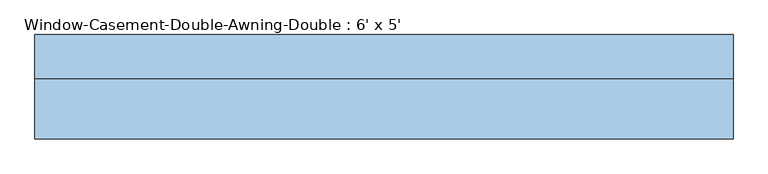
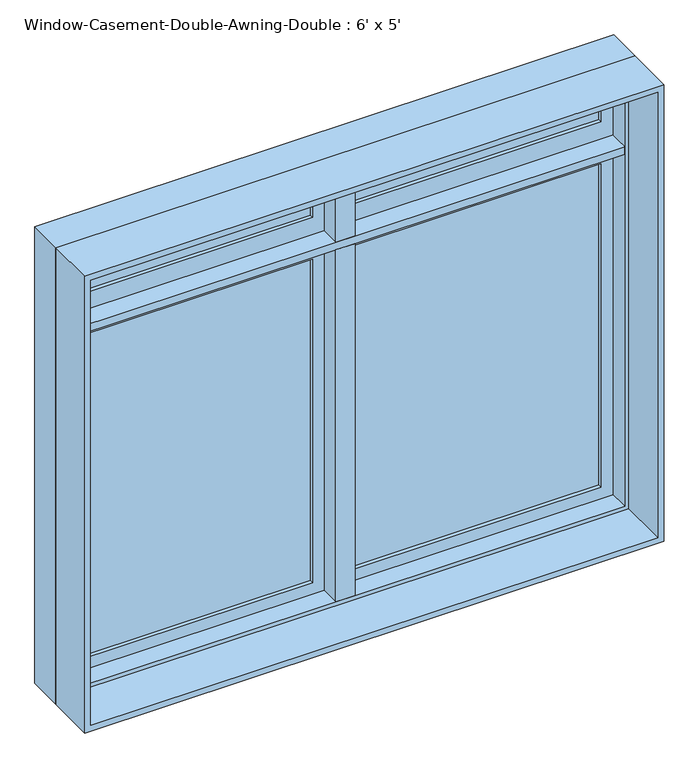
"""IFC4 building model written with IfcOpenShell, lengths in millimetres: window geometry, Window-Casement-Double-Awning-Double : 6' x 5'."""

from ifc_helpers import new_model, si_unit, frame, origin, place, context, project, spatial, polyline, outline, extrude, faceted_brep, source, transform, mapped, element, save


def window_casement_double_awning_double_6_x_5_2a8633dc(model_context):
    return source(origin(), model_context, "Body", "SolidModel", [
        faceted_brep([(882.65, 95.25, 2406.65), (882.65, 31.75, 2406.65), (-882.65, 31.75, 2406.65), (-882.65, 95.25, 2406.65), (901.7, 146.05, 2425.7), (901.7, 95.25, 2425.7), (-901.7, 95.25, 2425.7), (-901.7, 146.05, 2425.7), (914.4, 31.75, 2438.4), (914.4, 146.05, 2438.4), (-914.4, 146.05, 2438.4), (-914.4, 31.75, 2438.4), (-882.65, 31.75, 946.15), (-882.65, 95.25, 946.15), (-901.7, 95.25, 927.1), (-901.7, 146.05, 927.1), (-914.4, 146.05, 914.4), (-914.4, 31.75, 914.4), (882.65, 31.75, 946.15), (882.65, 95.25, 946.15), (901.7, 95.25, 927.1), (901.7, 146.05, 927.1), (914.4, 146.05, 914.4), (914.4, 31.75, 914.4)], [[[0, 1, 2, 3]], [[4, 5, 6, 7]], [[8, 9, 10, 11]], [[3, 2, 12, 13]], [[7, 6, 14, 15]], [[11, 10, 16, 17]], [[13, 12, 18, 19]], [[15, 14, 20, 21]], [[17, 16, 22, 23]], [[11, 17, 23, 8], [1, 18, 12, 2]], [[19, 18, 1, 0]], [[5, 20, 14, 6], [3, 13, 19, 0]], [[21, 20, 5, 4]], [[23, 22, 9, 8]], [[9, 22, 16, 10], [7, 15, 21, 4]]]),
        extrude(outline(polyline([(2438.4, -914.4), (914.4, -914.4), (914.4, 914.4), (2438.4, 914.4), (2438.4, -914.4)]), holes=[polyline([(2419.35, 895.35), (933.45, 895.35), (933.45, -895.35), (2419.35, -895.35), (2419.35, 895.35)])]), frame((0.0, -127.0, 0.0), z_axis=(0.0, 1.0, 0.0), x_axis=(0.0, 0.0, 1.0)), (0.0, 0.0, 1.0), 158.75),
        extrude(outline(polyline([(927.1, 901.7), (2120.9, 901.7), (2120.9, 9.525), (927.1, 9.525), (927.1, 901.7)]), holes=[polyline([(984.25, 66.675), (2063.75, 66.675), (2063.75, 844.55), (984.25, 844.55), (984.25, 66.675)])]), frame((0.0, 95.25, 0.0), z_axis=(0.0, 1.0, 0.0), x_axis=(0.0, 0.0, 1.0)), (0.0, 0.0, 1.0), 44.45),
        extrude(outline(polyline([(2120.9, -901.7), (927.1, -901.7), (927.1, -9.525), (2120.9, -9.525), (2120.9, -901.7)]), holes=[polyline([(2063.75, -66.675), (984.25, -66.675), (984.25, -844.55), (2063.75, -844.55), (2063.75, -66.675)])]), frame((0.0, 95.25, 0.0), z_axis=(0.0, 1.0, 0.0), x_axis=(0.0, 0.0, 1.0)), (0.0, 0.0, 1.0), 44.45),
        extrude(outline(polyline([(844.55, 127.0), (844.55, 120.65), (66.675, 120.65), (66.675, 127.0), (844.55, 127.0)])), frame((0.0, 0.0, 984.25), z_axis=(0.0, 0.0, 1.0), x_axis=(1.0, 0.0, 0.0)), (0.0, 0.0, 1.0), 1079.5),
        extrude(outline(polyline([(66.675, 107.95), (66.675, 114.3), (844.55, 114.3), (844.55, 107.95), (66.675, 107.95)])), frame((0.0, 0.0, 984.25), z_axis=(0.0, 0.0, 1.0), x_axis=(1.0, 0.0, 0.0)), (0.0, 0.0, 1.0), 1079.5),
        extrude(outline(polyline([(-66.675, 127.0), (-66.675, 120.65), (-844.55, 120.65), (-844.55, 127.0), (-66.675, 127.0)])), frame((0.0, 0.0, 984.25), z_axis=(0.0, 0.0, 1.0), x_axis=(1.0, 0.0, 0.0)), (0.0, 0.0, 1.0), 1079.5),
        extrude(outline(polyline([(-844.55, 107.95), (-844.55, 114.3), (-66.675, 114.3), (-66.675, 107.95), (-844.55, 107.95)])), frame((0.0, 0.0, 984.25), z_axis=(0.0, 0.0, 1.0), x_axis=(1.0, 0.0, 0.0)), (0.0, 0.0, 1.0), 1079.5),
        faceted_brep([(9.525, 146.05, 2120.9), (-9.525, 146.05, 2120.9), (-9.525, 95.25, 2120.9), (-30.1625, 95.25, 2120.9), (-30.1625, 31.75, 2120.9), (30.1625, 31.75, 2120.9), (30.1625, 95.25, 2120.9), (9.525, 95.25, 2120.9), (9.525, 146.05, 927.1), (9.525, 95.25, 927.1), (-9.525, 95.25, 927.1), (-9.525, 146.05, 927.1), (-9.525, 95.25, 946.15), (-30.1625, 95.25, 946.15), (-30.1625, 31.75, 946.15), (30.1625, 31.75, 946.15), (30.1625, 95.25, 946.15), (9.525, 95.25, 946.15)], [[[0, 1, 2, 3, 4, 5, 6, 7]], [[8, 9, 10, 11]], [[1, 0, 8, 11]], [[2, 1, 11, 10, 12]], [[3, 2, 12, 13]], [[4, 3, 13, 14]], [[5, 4, 14, 15]], [[6, 5, 15, 16]], [[7, 6, 16, 17]], [[0, 7, 17, 9, 8]], [[17, 12, 10, 9]], [[12, 17, 16, 15, 14, 13]]]),
        extrude(outline(polyline([(-66.675, 127.0), (-66.675, 120.65), (-844.55, 120.65), (-844.55, 127.0), (-66.675, 127.0)])), frame((0.0, 0.0, 2203.45), z_axis=(0.0, 0.0, 1.0), x_axis=(1.0, 0.0, 0.0)), (0.0, 0.0, 1.0), 165.1),
        extrude(outline(polyline([(-844.55, 107.95), (-844.55, 114.3), (-66.675, 114.3), (-66.675, 107.95), (-844.55, 107.95)])), frame((0.0, 0.0, 2203.45), z_axis=(0.0, 0.0, 1.0), x_axis=(1.0, 0.0, 0.0)), (0.0, 0.0, 1.0), 165.1),
        extrude(outline(polyline([(901.7, 146.05), (901.7, 95.25), (882.65, 95.25), (882.65, 31.75), (-882.65, 31.75), (-882.65, 95.25), (-901.7, 95.25), (-901.7, 146.05), (901.7, 146.05)])), frame((0.0, 0.0, 2120.9), z_axis=(0.0, 0.0, 1.0), x_axis=(1.0, 0.0, 0.0)), (0.0, 0.0, 1.0), 25.4),
        faceted_brep([(9.525, 95.25, 2425.7), (9.525, 146.05, 2425.7), (-9.525, 146.05, 2425.7), (-9.525, 95.25, 2425.7), (-9.525, 95.25, 2146.3), (-9.525, 146.05, 2146.3), (9.525, 146.05, 2146.3), (9.525, 95.25, 2146.3), (30.1625, 95.25, 2146.3), (30.1625, 31.75, 2146.3), (-30.1625, 31.75, 2146.3), (-30.1625, 95.25, 2146.3), (-30.1625, 95.25, 2406.65), (-9.525, 95.25, 2406.65), (-30.1625, 31.75, 2406.65), (30.1625, 31.75, 2406.65), (30.1625, 95.25, 2406.65), (9.525, 95.25, 2406.65)], [[[0, 1, 2, 3]], [[4, 5, 6, 7, 8, 9, 10, 11]], [[4, 11, 12, 13]], [[11, 10, 14, 12]], [[10, 9, 15, 14]], [[9, 8, 16, 15]], [[8, 7, 17, 16]], [[1, 0, 17, 7, 6]], [[2, 1, 6, 5]], [[3, 2, 5, 4, 13]], [[17, 13, 12, 14, 15, 16]], [[13, 17, 0, 3]]]),
        extrude(outline(polyline([(2425.7, 9.525), (2146.3, 9.525), (2146.3, 901.7), (2425.7, 901.7), (2425.7, 9.525)]), holes=[polyline([(2368.55, 844.55), (2203.45, 844.55), (2203.45, 66.675), (2368.55, 66.675), (2368.55, 844.55)])]), frame((0.0, 95.25, 0.0), z_axis=(0.0, 1.0, 0.0), x_axis=(0.0, 0.0, 1.0)), (0.0, 0.0, 1.0), 44.45),
        extrude(outline(polyline([(2146.3, -9.525), (2425.7, -9.525), (2425.7, -901.7), (2146.3, -901.7), (2146.3, -9.525)]), holes=[polyline([(2203.45, -844.55), (2368.55, -844.55), (2368.55, -66.675), (2203.45, -66.675), (2203.45, -844.55)])]), frame((0.0, 95.25, 0.0), z_axis=(0.0, 1.0, 0.0), x_axis=(0.0, 0.0, 1.0)), (0.0, 0.0, 1.0), 44.45),
        extrude(outline(polyline([(66.675, 127.0), (844.55, 127.0), (844.55, 120.65), (66.675, 120.65), (66.675, 127.0)])), frame((0.0, 0.0, 2203.45), z_axis=(0.0, 0.0, 1.0), x_axis=(1.0, 0.0, 0.0)), (0.0, 0.0, 1.0), 165.1),
        extrude(outline(polyline([(844.55, 107.95), (66.675, 107.95), (66.675, 114.3), (844.55, 114.3), (844.55, 107.95)])), frame((0.0, 0.0, 2203.45), z_axis=(0.0, 0.0, 1.0), x_axis=(1.0, 0.0, 0.0)), (0.0, 0.0, 1.0), 165.1),
    ])


if __name__ == "__main__":
    model = new_model("IFC4")
    model_context = context("Model", 3, world=origin())
    ifc_project = project(units=[si_unit("LENGTHUNIT", "METRE", prefix="MILLI")], contexts=[model_context])
    site = spatial("IfcSite", under=ifc_project)
    building = spatial("IfcBuilding", under=site)
    placement = place(None, origin())
    window_casement_double_awning_double_6_x_5_shape = window_casement_double_awning_double_6_x_5_2a8633dc(model_context)
    element("IfcWindow", 1, ObjectType="Window-Casement-Double-Awning-Double : 6' x 5'", at=placement, inside=building, context=model_context, shape_type="MappedRepresentation", body=[
        mapped(window_casement_double_awning_double_6_x_5_shape, transform((0.0, 0.0, 0.0), x_axis=(1.0, 0.0, 0.0), y_axis=(0.0, 1.0, 0.0), z_axis=(0.0, 0.0, 1.0))),
    ])
    save(model, "model.ifc")

# Revit data of these elements
# Type "Window-Casement-Double-Awning-Double : 6' x 5'"
#   Type Mark = "22"
#   Fire Rating = "0.5h"
#   Assembly Code = "B2020100"
#   Analytic Construction = "Double glazing - domestic"
#   Window Inset [instance default] = 0' - 0"
#   Wall Thickness [instance default] = 0' - 6"
#   Interior Wall Closure [instance default] = 0' - 2 1/4"
#   Half Width = 3' - 0"
#   Visual Light Transmittance = 0.81
#   Transom Height = 1' - 0"
#   Thermal Resistance (R) = 1.8146 (h·ft²·°F)/BTU
#   Solar Heat Gain Coefficient = 0.76
#   Rough Width = 6' - 0 1/2"
#   Rough Height = 5' - 0 1/2"
#   Open Window Height = 4' - 0"
#   Frame Extension [instance default] = 0' - 0 1/4"
#   Height = 5' - 0"
#   Heat Transfer Coefficient (U) = 0.5511 BTU/(h·ft²·°F)
#   Exterior Wall Closure [instance default] = 0' - 1 1/4"
#   Extension Jamb [instance default] = 0' - 2 1/4"
#   Default Sill Height = 3' - 0"
#   Width = 6' - 0"
#   Top Muntin Visibility = yes
#   Bottom Muntin Visibility = yes
#   Interior Trim Visibility [instance default] = yes
#   Exterior Trim Visibility [instance default] = yes
#   Extension Jamb Visibility [instance default] = yes
#   Interior Trim Material = Wood - Stained
#   Muntin Pattern = Muntin Pattern_2x2 : Muntin Pattern_2x2
#   Interior Trim = Trim-Window-Interior-Flat : Picture Frame
#   Interior Frame Material = Wood - Stained
#   Glass Panel Material = Glass
#   Exterior Trim Material = Clad - White
#   Exterior Trim = Trim-Window-Exterior-Flat : with Sill
#   Exterior Frame Material = Clad - White
#   Wall Closure = (empty or 0)
# Element 1 (IfcWindow, "Window-Casement-Double-Awning-Double : 6' x 5'")
#   Wall Thickness = 0' - 10"
#   Extension Jamb = 0' - 6 1/4"
#   Materials on its faces: "Wood - Stained", "Glass", "Clad - White"
# Materials
#   "Wood - Stained": class "Wood", colour RGB 224 178 126, transparency 0, Cost = 0
#   "Glass": class "Glass", colour RGB 0 128 192, transparency 0.75, Description = "Soda Lime Glass", Cost = 0
#   "Clad - White": class "Wood", colour RGB 242 242 238, transparency 0, Cost = 0
